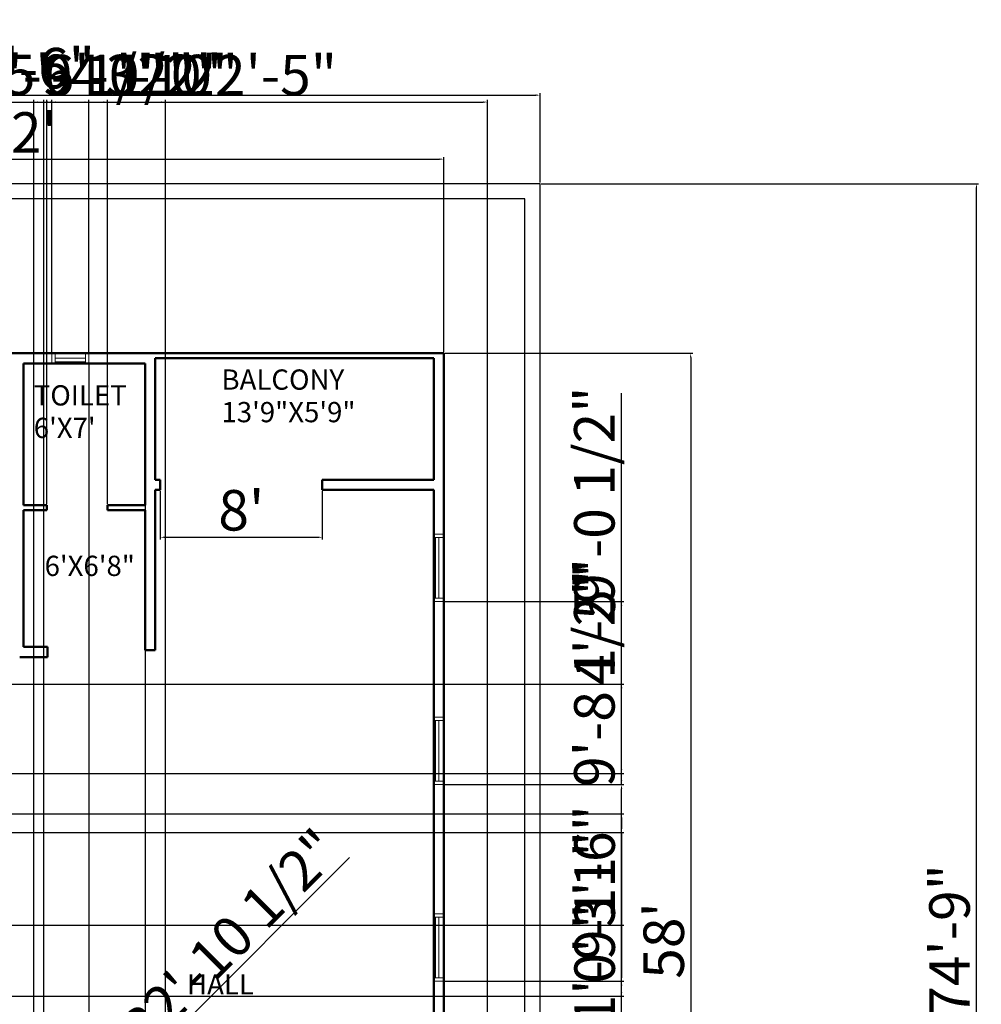
# Model space of a CAD drawing. Units: inches. Extents: x 2047 to 3023, y 479 to 1545.
# Tile 3 of 3: x 2454 to 3023, y 961 to 1545. Entities that reach past the tile are written whole.
import ezdxf

# ---------------------------------------------------------------- set-up
doc = ezdxf.new("R2010")
doc.units = ezdxf.units.IN
for name, color, linetype, lineweight in [('A-ANNO-DIMS', 2, 'Continuous', 18), ('A-AREA-IDEN', 7, 'Continuous', 25), ('A-GLAZ', 4, 'Continuous', 18), ('A-WALL', 7, 'Continuous', 50), ('C-PROP', 8, 'Continuous', 30)]:
    doc.layers.add(name, color=color, linetype=linetype, lineweight=lineweight)
doc.styles.get("Standard").update_dxf_attribs({"font": 'arial.ttf'})
doc.dimstyles.new('ISO-25', dxfattribs={"dimtxt": 24, "dimasz": 2.5, "dimexe": 1.25, "dimexo": 0.625, "dimtad": 1, "dimdec": 1, "dimlunit": 3, "dimtxsty": 'Standard', "dimcen": 2.5, "dimadec": 0, "dimazin": 0, "dimtfac": 1, "dimtdec": 1, "dimtmove": 0, "dimatfit": 3, "dimfxl": 1, "dimarcsym": 0})

# ---------------------------------------------------------------- blocks, each defined once
blk = doc.blocks.new('*D3')
at = {"layer": 'A-ANNO-DIMS', "color": 0, "lineweight": -2, "transparency": 16777216}
for p, q in [((2762.53, 1447.48), (3021.8, 1447.48)), ((3020.55, 552.98), (3020.55, 1444.98)), ((2762.53, 550.48), (3021.8, 550.48))]:
    blk.add_line(p, q, dxfattribs=at)
at = {"layer": 'A-ANNO-DIMS', "color": 0, "transparency": 16777216}
for points in [[(3020.13, 1444.98), (3020.96, 1444.98), (3020.55, 1447.48)], [(3020.13, 552.98), (3020.96, 552.98), (3020.55, 550.48)]]:
    blk.add_solid(points, dxfattribs=at)
at = {"layer": 'Defpoints', "color": 0, "transparency": 16777216}
for p in [(2761.91, 1447.48), (3020.55, 1447.48), (2761.91, 550.48)]:
    blk.add_point(p, dxfattribs=at)
at = {"layer": 'A-ANNO-DIMS', "color": 0, "transparency": 16777216, "insert": (3007.67, 998.98), "char_height": 24, "attachment_point": 5, "rotation": 90}
blk.add_mtext('74\'-9"', dxfattribs=at)
blk = doc.blocks.new('*D4')
at = {"layer": 'A-ANNO-DIMS', "color": 0, "lineweight": -2, "transparency": 16777216}
for p, q in [((2143.91, 1448.11), (2143.91, 1501.19)), ((2146.41, 1499.94), (2759.41, 1499.94)), ((2761.91, 1448.11), (2761.91, 1501.19))]:
    blk.add_line(p, q, dxfattribs=at)
at = {"layer": 'A-ANNO-DIMS', "color": 0, "transparency": 16777216}
for points in [[(2146.41, 1500.36), (2146.41, 1499.52), (2143.91, 1499.94)], [(2759.41, 1500.36), (2759.41, 1499.52), (2761.91, 1499.94)]]:
    blk.add_solid(points, dxfattribs=at)
at = {"layer": 'Defpoints', "color": 0, "transparency": 16777216}
for p in [(2761.91, 1499.94), (2143.91, 1447.48), (2761.91, 1447.48)]:
    blk.add_point(p, dxfattribs=at)
at = {"layer": 'A-ANNO-DIMS', "color": 0, "transparency": 16777216, "insert": (2452.91, 1512.82), "char_height": 24, "attachment_point": 5}
blk.add_mtext('51\'-6"', dxfattribs=at)
blk = doc.blocks.new('*D5')
at = {"layer": 'A-ANNO-DIMS', "color": 0, "lineweight": -2, "transparency": 16777216}
for p, q in [((2200.91, 1347.61), (2200.91, 1463.28)), ((2203.41, 1462.03), (2702.41, 1462.03)), ((2704.91, 1347.61), (2704.91, 1463.28))]:
    blk.add_line(p, q, dxfattribs=at)
at = {"layer": 'A-ANNO-DIMS', "color": 0, "transparency": 16777216}
for points in [[(2203.41, 1462.44), (2203.41, 1461.61), (2200.91, 1462.03)], [(2702.41, 1462.44), (2702.41, 1461.61), (2704.91, 1462.03)]]:
    blk.add_solid(points, dxfattribs=at)
at = {"layer": 'Defpoints', "color": 0, "transparency": 16777216}
for p in [(2704.91, 1462.03), (2200.91, 1346.98), (2704.91, 1346.98)]:
    blk.add_point(p, dxfattribs=at)
at = {"layer": 'A-ANNO-DIMS', "color": 0, "transparency": 16777216, "insert": (2452.91, 1474.7), "char_height": 24, "attachment_point": 5}
blk.add_mtext("42'", dxfattribs=at)
blk = doc.blocks.new('*D6')
at = {"layer": 'A-ANNO-DIMS', "color": 0, "lineweight": -2, "transparency": 16777216}
for p, q in [((2705.53, 1346.98), (2852.44, 1346.98)), ((2851.19, 1344.48), (2851.19, 653.48)), ((2705.53, 650.98), (2852.44, 650.98))]:
    blk.add_line(p, q, dxfattribs=at)
at = {"layer": 'A-ANNO-DIMS', "color": 0, "transparency": 16777216}
for points in [[(2850.77, 1344.48), (2851.6, 1344.48), (2851.19, 1346.98)], [(2850.77, 653.48), (2851.6, 653.48), (2851.19, 650.98)]]:
    blk.add_solid(points, dxfattribs=at)
at = {"layer": 'Defpoints', "color": 0, "transparency": 16777216}
for p in [(2704.91, 1346.98), (2704.91, 650.98), (2851.19, 650.98)]:
    blk.add_point(p, dxfattribs=at)
at = {"layer": 'A-ANNO-DIMS', "color": 0, "transparency": 16777216, "insert": (2838.31, 998.98), "char_height": 24, "attachment_point": 5, "rotation": 90}
blk.add_mtext("58'", dxfattribs=at)
blk = doc.blocks.new('*D9')
at = {"layer": 'A-ANNO-DIMS', "color": 0, "lineweight": -2, "transparency": 16777216}
for p, q in [((2536.91, 1265.36), (2536.91, 1236.68)), ((2632.91, 1265.36), (2632.91, 1236.68)), ((2539.41, 1237.93), (2630.41, 1237.93))]:
    blk.add_line(p, q, dxfattribs=at)
at = {"layer": 'A-ANNO-DIMS', "color": 0, "transparency": 16777216}
for points in [[(2539.41, 1238.35), (2539.41, 1237.52), (2536.91, 1237.93)], [(2630.41, 1238.35), (2630.41, 1237.52), (2632.91, 1237.93)]]:
    blk.add_solid(points, dxfattribs=at)
at = {"layer": 'Defpoints', "color": 0, "transparency": 16777216}
for p in [(2536.91, 1265.98), (2632.91, 1265.98), (2632.91, 1237.93)]:
    blk.add_point(p, dxfattribs=at)
at = {"layer": 'A-ANNO-DIMS', "color": 0, "transparency": 16777216, "insert": (2584.91, 1250.81), "char_height": 24, "attachment_point": 5}
blk.add_mtext("8'", dxfattribs=at)
blk = doc.blocks.new('WIN-36IN-6IN-FRAME')
for p, q in [((0, 6), (0, 0)), ((38, 6), (2, 6)), ((2, 6), (2, 0)), ((38, 0), (38, 6)), ((40, 0), (40, 6)), ((38, 5), (2, 5)), ((38, 3), (2, 3)), ((2, 0), (38, 0))]:
    blk.add_line(p, q)
blk = doc.blocks.new('*D24')
at = {"layer": 'A-ANNO-DIMS', "color": 0, "lineweight": -2, "transparency": 16777216}
for p, q in [((2461.91, 594.24), (2461.91, 1497.08)), ((2464.41, 1495.83), (2728.27, 1495.83)), ((2730.77, 594.24), (2730.77, 1497.08))]:
    blk.add_line(p, q, dxfattribs=at)
at = {"layer": 'A-ANNO-DIMS', "color": 0, "transparency": 16777216}
for points in [[(2464.41, 1496.25), (2464.41, 1495.41), (2461.91, 1495.83)], [(2728.27, 1496.25), (2728.27, 1495.41), (2730.77, 1495.83)]]:
    blk.add_solid(points, dxfattribs=at)
at = {"layer": 'Defpoints', "color": 0, "transparency": 16777216}
for p in [(2730.77, 1495.83), (2461.91, 593.62), (2730.77, 593.62)]:
    blk.add_point(p, dxfattribs=at)
at = {"layer": 'A-ANNO-DIMS', "color": 0, "transparency": 16777216, "insert": (2596.34, 1508.71), "char_height": 24, "attachment_point": 5}
blk.add_mtext('22\'-5"', dxfattribs=at)
blk = doc.blocks.new('*D32')
at = {"layer": 'A-ANNO-DIMS', "color": 0, "lineweight": -2, "transparency": 16777216}
for p, q in [((2705.53, 974.8), (2811.51, 974.8)), ((2810.26, 863.48), (2810.26, 972.3)), ((2699.53, 860.98), (2811.51, 860.98))]:
    blk.add_line(p, q, dxfattribs=at)
at = {"layer": 'A-ANNO-DIMS', "color": 0, "transparency": 16777216}
for points in [[(2809.84, 972.3), (2810.67, 972.3), (2810.26, 974.8)], [(2809.84, 863.48), (2810.67, 863.48), (2810.26, 860.98)]]:
    blk.add_solid(points, dxfattribs=at)
at = {"layer": 'Defpoints', "color": 0, "transparency": 16777216}
for p in [(2704.91, 974.8), (2810.26, 974.8), (2698.91, 860.98)]:
    blk.add_point(p, dxfattribs=at)
at = {"layer": 'A-ANNO-DIMS', "color": 0, "transparency": 16777216, "insert": (2797.38, 917.89), "char_height": 24, "attachment_point": 5, "rotation": 90}
blk.add_mtext('9\'-6"', dxfattribs=at)
blk = doc.blocks.new('*D33')
at = {"layer": 'A-ANNO-DIMS', "color": 0, "lineweight": -2, "transparency": 16777216}
for p, q in [((2810.26, 1091.4), (2810.26, 1214.87)), ((2705.53, 1091.4), (2811.51, 1091.4)), ((2810.26, 977.3), (2810.26, 1088.9)), ((2705.53, 974.8), (2811.51, 974.8))]:
    blk.add_line(p, q, dxfattribs=at)
at = {"layer": 'A-ANNO-DIMS', "color": 0, "transparency": 16777216}
for points in [[(2809.84, 1088.9), (2810.67, 1088.9), (2810.26, 1091.4)], [(2809.84, 977.3), (2810.67, 977.3), (2810.26, 974.8)]]:
    blk.add_solid(points, dxfattribs=at)
at = {"layer": 'Defpoints', "color": 0, "transparency": 16777216}
for p in [(2704.91, 1091.4), (2810.26, 1091.4), (2704.91, 974.8)]:
    blk.add_point(p, dxfattribs=at)
at = {"layer": 'A-ANNO-DIMS', "color": 0, "transparency": 16777216, "insert": (2797.22, 1154.38), "char_height": 24, "attachment_point": 5, "rotation": 90}
blk.add_mtext('9\'-8 1/2"', dxfattribs=at)
blk = doc.blocks.new('*D34')
at = {"layer": 'A-ANNO-DIMS', "color": 0, "lineweight": -2, "transparency": 16777216}
for p, q in [((2810.26, 1199.82), (2810.26, 1323.3)), ((2705.53, 1199.82), (2811.51, 1199.82)), ((2810.26, 1093.9), (2810.26, 1197.32)), ((2705.53, 1091.4), (2811.51, 1091.4))]:
    blk.add_line(p, q, dxfattribs=at)
at = {"layer": 'A-ANNO-DIMS', "color": 0, "transparency": 16777216}
for points in [[(2809.84, 1197.32), (2810.67, 1197.32), (2810.26, 1199.82)], [(2809.84, 1093.9), (2810.67, 1093.9), (2810.26, 1091.4)]]:
    blk.add_solid(points, dxfattribs=at)
at = {"layer": 'Defpoints', "color": 0, "transparency": 16777216}
for p in [(2704.91, 1199.82), (2810.26, 1199.82), (2704.91, 1091.4)]:
    blk.add_point(p, dxfattribs=at)
at = {"layer": 'A-ANNO-DIMS', "color": 0, "transparency": 16777216, "insert": (2797.22, 1262.81), "char_height": 24, "attachment_point": 5, "rotation": 90}
blk.add_mtext('9\'-0 1/2"', dxfattribs=at)
blk = doc.blocks.new('*D38')
at = {"layer": 'A-ANNO-DIMS', "color": 0, "lineweight": -2, "transparency": 16777216}
for p, q in [((2494.55, 1340.36), (2494.55, 500.88)), ((2527.91, 1340.36), (2527.91, 500.88)), ((2497.05, 502.13), (2525.41, 502.13)), ((2527.91, 502.13), (2651.79, 502.13))]:
    blk.add_line(p, q, dxfattribs=at)
at = {"layer": 'A-ANNO-DIMS', "color": 0, "transparency": 16777216}
for points in [[(2497.05, 502.55), (2497.05, 501.71), (2494.55, 502.13)], [(2525.41, 502.55), (2525.41, 501.71), (2527.91, 502.13)]]:
    blk.add_solid(points, dxfattribs=at)
at = {"layer": 'Defpoints', "color": 0, "transparency": 16777216}
for p in [(2494.55, 1340.98), (2527.91, 1340.98), (2527.91, 502.13)]:
    blk.add_point(p, dxfattribs=at)
at = {"layer": 'A-ANNO-DIMS', "color": 0, "transparency": 16777216, "insert": (2591.1, 515.16), "char_height": 24, "attachment_point": 5}
blk.add_mtext('2\'-9 1/2"', dxfattribs=at)
blk = doc.blocks.new('*D39')
at = {"layer": 'A-ANNO-DIMS', "color": 0, "lineweight": -2, "transparency": 16777216}
for p, q in [((2472.55, 1347.61), (2472.55, 1497.08)), ((2475.05, 1495.83), (2492.05, 1495.83)), ((2494.55, 1347.61), (2494.55, 1497.08)), ((2494.55, 1495.83), (2578.49, 1495.83))]:
    blk.add_line(p, q, dxfattribs=at)
at = {"layer": 'A-ANNO-DIMS', "color": 0, "transparency": 16777216}
for points in [[(2475.05, 1496.25), (2475.05, 1495.41), (2472.55, 1495.83)], [(2492.05, 1496.25), (2492.05, 1495.41), (2494.55, 1495.83)]]:
    blk.add_solid(points, dxfattribs=at)
at = {"layer": 'Defpoints', "color": 0, "transparency": 16777216}
for p in [(2494.55, 1495.83), (2472.55, 1346.98), (2494.55, 1346.98)]:
    blk.add_point(p, dxfattribs=at)
at = {"layer": 'A-ANNO-DIMS', "color": 0, "transparency": 16777216, "insert": (2537.77, 1508.71), "char_height": 24, "attachment_point": 5}
blk.add_mtext('1\'-10"', dxfattribs=at)
blk = doc.blocks.new('*D41')
at = {"layer": 'A-ANNO-DIMS', "color": 0, "lineweight": -2, "transparency": 16777216}
for p, q in [((2381.88, 867.61), (2381.88, 1497.08)), ((2384.38, 1495.83), (2443.66, 1495.83)), ((2446.16, 867.61), (2446.16, 1497.08)), ((2446.16, 1495.83), (2569.64, 1495.83))]:
    blk.add_line(p, q, dxfattribs=at)
at = {"layer": 'A-ANNO-DIMS', "color": 0, "transparency": 16777216}
for points in [[(2384.38, 1496.25), (2384.38, 1495.41), (2381.88, 1495.83)], [(2443.66, 1496.25), (2443.66, 1495.41), (2446.16, 1495.83)]]:
    blk.add_solid(points, dxfattribs=at)
at = {"layer": 'Defpoints', "color": 0, "transparency": 16777216}
for p in [(2446.16, 1495.83), (2381.88, 866.98), (2446.16, 866.98)]:
    blk.add_point(p, dxfattribs=at)
at = {"layer": 'A-ANNO-DIMS', "color": 0, "transparency": 16777216, "insert": (2509.15, 1508.86), "char_height": 24, "attachment_point": 5}
blk.add_mtext('5\'-4 1/2"', dxfattribs=at)
blk = doc.blocks.new('*D42')
at = {"layer": 'A-ANNO-DIMS', "color": 0, "lineweight": -2, "transparency": 16777216}
for p, q in [((2810.26, 950.97), (2810.26, 1016.25)), ((2362.53, 950.97), (2811.51, 950.97)), ((2810.26, 932.42), (2810.26, 948.47)), ((2362.53, 929.92), (2811.51, 929.92))]:
    blk.add_line(p, q, dxfattribs=at)
at = {"layer": 'A-ANNO-DIMS', "color": 0, "transparency": 16777216}
for points in [[(2809.84, 948.47), (2810.67, 948.47), (2810.26, 950.97)], [(2809.84, 932.42), (2810.67, 932.42), (2810.26, 929.92)]]:
    blk.add_solid(points, dxfattribs=at)
at = {"layer": 'Defpoints', "color": 0, "transparency": 16777216}
for p in [(2361.91, 950.97), (2810.26, 950.97), (2361.91, 929.92)]:
    blk.add_point(p, dxfattribs=at)
at = {"layer": 'A-ANNO-DIMS', "color": 0, "transparency": 16777216, "insert": (2797.38, 984.86), "char_height": 24, "attachment_point": 5, "rotation": 90}
blk.add_mtext('1\'-9"', dxfattribs=at)
blk = doc.blocks.new('*D46')
at = {"layer": 'A-ANNO-DIMS', "color": 0, "lineweight": -2, "transparency": 16777216}
for p, q in [((2810.26, 1007.98), (2810.26, 1075.51)), ((2360.53, 1007.98), (2811.51, 1007.98)), ((2810.26, 968.48), (2810.26, 1005.48)), ((2360.53, 965.98), (2811.51, 965.98))]:
    blk.add_line(p, q, dxfattribs=at)
at = {"layer": 'A-ANNO-DIMS', "color": 0, "transparency": 16777216}
for points in [[(2809.84, 1005.48), (2810.67, 1005.48), (2810.26, 1007.98)], [(2809.84, 968.48), (2810.67, 968.48), (2810.26, 965.98)]]:
    blk.add_solid(points, dxfattribs=at)
at = {"layer": 'Defpoints', "color": 0, "transparency": 16777216}
for p in [(2359.91, 1007.98), (2810.26, 1007.98), (2359.91, 965.98)]:
    blk.add_point(p, dxfattribs=at)
at = {"layer": 'A-ANNO-DIMS', "color": 0, "transparency": 16777216, "insert": (2797.37, 1043), "char_height": 24, "attachment_point": 5, "rotation": 90}
blk.add_mtext('3\'-6"', dxfattribs=at)
blk = doc.blocks.new('*D47')
at = {"layer": 'A-ANNO-DIMS', "color": 0, "lineweight": -2, "transparency": 16777216}
for p, q in [((2810.26, 1150.98), (2810.26, 1219.49)), ((2294.53, 1150.98), (2811.51, 1150.98)), ((2810.26, 1100.48), (2810.26, 1148.48)), ((2294.53, 1097.98), (2811.51, 1097.98))]:
    blk.add_line(p, q, dxfattribs=at)
at = {"layer": 'A-ANNO-DIMS', "color": 0, "transparency": 16777216}
for points in [[(2809.84, 1148.48), (2810.67, 1148.48), (2810.26, 1150.98)], [(2809.84, 1100.48), (2810.67, 1100.48), (2810.26, 1097.98)]]:
    blk.add_solid(points, dxfattribs=at)
at = {"layer": 'Defpoints', "color": 0, "transparency": 16777216}
for p in [(2293.91, 1150.98), (2810.26, 1150.98), (2293.91, 1097.98)]:
    blk.add_point(p, dxfattribs=at)
at = {"layer": 'A-ANNO-DIMS', "color": 0, "transparency": 16777216, "insert": (2797.43, 1186.49), "char_height": 24, "attachment_point": 5, "rotation": 90}
blk.add_mtext('4\'-5"', dxfattribs=at)
blk = doc.blocks.new('*D49')
at = {"layer": 'A-ANNO-DIMS', "color": 0, "lineweight": -2, "transparency": 16777216}
for p, q in [((2250.53, 1073.98), (2811.51, 1073.98)), ((2810.26, 1071.48), (2810.26, 1065.48)), ((2250.53, 1062.98), (2811.51, 1062.98)), ((2810.26, 1062.98), (2810.26, 976.79))]:
    blk.add_line(p, q, dxfattribs=at)
at = {"layer": 'A-ANNO-DIMS', "color": 0, "transparency": 16777216}
for points in [[(2809.84, 1071.48), (2810.67, 1071.48), (2810.26, 1073.98)], [(2809.84, 1065.48), (2810.67, 1065.48), (2810.26, 1062.98)]]:
    blk.add_solid(points, dxfattribs=at)
at = {"layer": 'Defpoints', "color": 0, "transparency": 16777216}
for p in [(2249.91, 1073.98), (2249.91, 1062.98), (2810.26, 1062.98)]:
    blk.add_point(p, dxfattribs=at)
at = {"layer": 'A-ANNO-DIMS', "color": 0, "transparency": 16777216, "insert": (2797.38, 1018.63), "char_height": 24, "attachment_point": 5, "rotation": 90}
blk.add_mtext('0\'-11"', dxfattribs=at)
blk = doc.blocks.new('*D50')
at = {"layer": 'A-ANNO-DIMS', "color": 0, "lineweight": -2, "transparency": 16777216}
for p, q in [((2311.99, 1173.61), (2311.99, 1497.08)), ((2314.49, 1495.83), (2427.04, 1495.83)), ((2429.54, 1173.61), (2429.54, 1497.08)), ((2429.54, 1495.83), (2553.01, 1495.83))]:
    blk.add_line(p, q, dxfattribs=at)
at = {"layer": 'A-ANNO-DIMS', "color": 0, "transparency": 16777216}
for points in [[(2314.49, 1496.25), (2314.49, 1495.41), (2311.99, 1495.83)], [(2427.04, 1496.25), (2427.04, 1495.41), (2429.54, 1495.83)]]:
    blk.add_solid(points, dxfattribs=at)
at = {"layer": 'Defpoints', "color": 0, "transparency": 16777216}
for p in [(2429.54, 1495.83), (2311.99, 1172.98), (2429.54, 1172.98)]:
    blk.add_point(p, dxfattribs=at)
at = {"layer": 'A-ANNO-DIMS', "color": 0, "transparency": 16777216, "insert": (2492.53, 1508.86), "char_height": 24, "attachment_point": 5}
blk.add_mtext('9\'-9 1/2"', dxfattribs=at)
blk = doc.blocks.new('*D51')
at = {"layer": 'A-ANNO-DIMS', "color": 0, "lineweight": -2, "transparency": 16777216}
for p, q in [((2467.91, 903.61), (2467.91, 1497.08)), ((2470.41, 1495.83), (2537.41, 1495.83)), ((2539.91, 903.61), (2539.91, 1497.08))]:
    blk.add_line(p, q, dxfattribs=at)
at = {"layer": 'A-ANNO-DIMS', "color": 0, "transparency": 16777216}
for points in [[(2470.41, 1496.25), (2470.41, 1495.41), (2467.91, 1495.83)], [(2537.41, 1496.25), (2537.41, 1495.41), (2539.91, 1495.83)]]:
    blk.add_solid(points, dxfattribs=at)
at = {"layer": 'Defpoints', "color": 0, "transparency": 16777216}
for p in [(2539.91, 1495.83), (2467.91, 902.98), (2539.91, 902.98)]:
    blk.add_point(p, dxfattribs=at)
at = {"layer": 'A-ANNO-DIMS', "color": 0, "transparency": 16777216, "insert": (2503.91, 1508.71), "char_height": 24, "attachment_point": 5}
blk.add_mtext('6\'-0"', dxfattribs=at)
blk = doc.blocks.new('*D52')
at = {"layer": 'A-ANNO-DIMS', "color": 0, "lineweight": -2, "transparency": 16777216}
for p, q in [((2469.68, 1257.61), (2469.68, 1497.08)), ((2472.18, 1495.83), (2503.18, 1495.83)), ((2505.68, 1257.61), (2505.68, 1497.08)), ((2505.68, 1495.83), (2573.21, 1495.83))]:
    blk.add_line(p, q, dxfattribs=at)
at = {"layer": 'A-ANNO-DIMS', "color": 0, "transparency": 16777216}
for points in [[(2472.18, 1496.25), (2472.18, 1495.41), (2469.68, 1495.83)], [(2503.18, 1496.25), (2503.18, 1495.41), (2505.68, 1495.83)]]:
    blk.add_solid(points, dxfattribs=at)
at = {"layer": 'Defpoints', "color": 0, "transparency": 16777216}
for p in [(2505.68, 1495.83), (2469.68, 1256.98), (2505.68, 1256.98)]:
    blk.add_point(p, dxfattribs=at)
at = {"layer": 'A-ANNO-DIMS', "color": 0, "transparency": 16777216, "insert": (2540.69, 1508.72), "char_height": 24, "attachment_point": 5}
blk.add_mtext('3\'-0"', dxfattribs=at)
blk = doc.blocks.new('*D54')
at = {"layer": 'A-ANNO-DIMS', "color": 0, "lineweight": -2, "transparency": 16777216}
for p, q in [((2649.08, 1048.15), (2495.59, 894.67)), ((2469.41, 868.48), (2493.83, 892.9))]:
    blk.add_line(p, q, dxfattribs=at)
at = {"layer": 'A-ANNO-DIMS', "color": 0, "transparency": 16777216}
blk.add_solid([(2495.3, 894.96), (2495.89, 894.37), (2493.83, 892.9)], dxfattribs=at)
at = {"layer": 'Defpoints', "color": 0, "transparency": 16777216}
for p in [(2493.83, 892.9), (2469.41, 868.48)]:
    blk.add_point(p, dxfattribs=at)
at = {"layer": 'A-ANNO-DIMS', "color": 0, "transparency": 16777216, "insert": (2564.01, 981.51), "char_height": 24, "attachment_point": 5, "rotation": 44.99969}
blk.add_mtext('2X R2\'-10 1/2"', dxfattribs=at)

msp = doc.modelspace()

# ---------------------------------------------------------------- linework, layer by layer
at = {"layer": 'A-GLAZ'}
for p, q in [((2472.55, 1346.98), (2472.55, 1340.98)), ((2492.55, 1346.98), (2474.55, 1346.98)), ((2474.55, 1346.98), (2474.55, 1340.98)), ((2492.55, 1343.98), (2474.55, 1343.98)), ((2492.55, 1340.98), (2492.55, 1346.98)), ((2494.55, 1340.98), (2494.55, 1346.98)), ((2492.55, 1341.98), (2474.55, 1341.98)), ((2474.55, 1340.98), (2492.55, 1340.98))]:
    msp.add_line(p, q, dxfattribs=at)
at = {"layer": 'A-WALL'}
for p, q in [((2704.91, 1346.98), (2248.87, 1346.98)), ((2698.91, 1343.98), (2533.91, 1343.98)), ((2533.91, 1271.98), (2533.91, 1343.98)), ((2698.91, 1271.98), (2698.91, 1343.98)), ((2704.91, 650.98), (2704.91, 1346.98)), ((2527.91, 1340.98), (2455.91, 1340.98)), ((2455.91, 1256.98), (2455.91, 1340.98)), ((2455.91, 1256.98), (2455.91, 1340.98)), ((2527.91, 1256.98), (2527.91, 1340.98)), ((2536.91, 1271.98), (2533.91, 1271.98)), ((2536.91, 1271.98), (2536.91, 1265.98)), ((2698.91, 1271.98), (2632.91, 1271.98)), ((2632.91, 1271.98), (2632.91, 1265.98)), ((2533.91, 1170.98), (2533.91, 1265.98)), ((2536.91, 1265.98), (2533.91, 1265.98)), ((2698.91, 1265.98), (2632.91, 1265.98)), ((2698.91, 866.98), (2698.91, 1265.98)), ((2469.68, 1256.98), (2455.91, 1256.98)), ((2469.68, 1256.98), (2469.68, 1253.98)), ((2527.91, 1256.98), (2505.68, 1256.98)), ((2505.68, 1256.98), (2505.68, 1253.98)), ((2455.91, 1172.98), (2455.91, 1253.98)), ((2469.68, 1253.98), (2455.91, 1253.98)), ((2527.91, 1253.98), (2505.68, 1253.98)), ((2527.91, 1173.98), (2527.91, 1253.98)), ((2470.07, 1172.98), (2455.91, 1172.98)), ((2470.07, 1172.98), (2470.07, 1170.98)), ((2527.91, 1173.98), (2527.91, 1170.98)), ((2470.07, 1170.98), (2470.07, 1166.97)), ((2527.91, 1170.98), (2533.91, 1170.98)), ((2453.57, 1166.97), (2470.07, 1166.97))]:
    msp.add_line(p, q, dxfattribs=at)
at = {"layer": 'C-PROP'}
for points in [[(2692.81, 550.48), (2761.91, 550.48), (2761.91, 1447.48), (2143.91, 1447.48), (2143.91, 550.48), (2554.81, 550.48)], [(2692.81, 559.48), (2752.91, 559.48), (2752.91, 1438.48), (2152.91, 1438.48), (2152.91, 559.48), (2554.81, 559.48)]]:
    msp.add_lwpolyline(points, dxfattribs=at)

# ---------------------------------------------------------------- block references
at = {"layer": 'A-GLAZ'}
for p, rotation in [((2704.91, 1199.82), 90.00000000000095), ((2704.91, 1091.4), 90.00000000000115), ((2704.91, 974.8), 90.00000000000115)]:
    msp.add_blockref('WIN-36IN-6IN-FRAME', p, dxfattribs=dict(at, rotation=rotation))

# ---------------------------------------------------------------- texts
at = {"layer": 'A-AREA-IDEN'}
for s, p in [('BALCONY', (2573.13, 1325.38)), ('TOILET', (2461.92, 1316.03)), ('13\'9"X5\'9"', (2573.13, 1306.1)), ("6'X7'", (2461.92, 1296.76)), ('6\'X6\'8"', (2468.34, 1214.99)), ('HALL', (2552.73, 967.01))]:
    msp.add_text(s, height=12, dxfattribs=at).set_placement(p)

# ---------------------------------------------------------------- dimensions: what is measured, and where the dimension line sits
at = {"layer": 'A-ANNO-DIMS'}
for base, p1, p2, override, picture, middle in [((2429.5398, 1495.8302), (2311.9877, 1172.9802), (2429.5398, 1172.9802), {"dimdec": 1, "dimlfac": 1, "dimrnd": 0, "dimzin": 1, "dimdsep": 46, "dimlunit": 4, "dimfrac": 2}, '*D50', (2492.5257, 1508.8645)), ((2446.16, 1495.83), (2381.88, 866.98), (2446.16, 866.98), {"dimdec": 1, "dimlfac": 1, "dimrnd": 0, "dimzin": 1, "dimdsep": 46, "dimlunit": 4, "dimfrac": 2}, '*D41', (2509.15, 1508.86)), ((2761.91, 1499.94), (2143.91, 1447.48), (2761.91, 1447.48), {"dimclrd": 0, "dimclre": 0, "dimclrt": 0}, '*D4', (2452.91, 1512.82)), ((2730.77, 1495.83), (2461.91, 593.62), (2730.77, 593.62), {"dimdec": 1, "dimlfac": 1, "dimrnd": 0, "dimzin": 1, "dimdsep": 46, "dimlunit": 4, "dimfrac": 2}, '*D24', (2596.34, 1508.71)), ((2539.91, 1495.83), (2467.91, 902.98), (2539.91, 902.98), {"dimdec": 1, "dimlfac": 1, "dimrnd": 0, "dimzin": 1, "dimdsep": 46, "dimlunit": 4, "dimfrac": 2}, '*D51', (2503.91, 1508.71)), ((2505.68, 1495.83), (2469.68, 1256.98), (2505.68, 1256.98), {"dimdec": 1, "dimlfac": 1, "dimrnd": 0, "dimzin": 1, "dimdsep": 46, "dimlunit": 4, "dimfrac": 2}, '*D52', (2540.69, 1508.72)), ((2494.55, 1495.83), (2472.55, 1346.98), (2494.55, 1346.98), {"dimdec": 1, "dimlfac": 1, "dimrnd": 0, "dimzin": 1, "dimdsep": 46, "dimlunit": 4, "dimfrac": 2}, '*D39', (2537.77, 1508.71)), ((2704.91, 1462.03), (2200.91, 1346.98), (2704.91, 1346.98), {"dimclrd": 0, "dimclre": 0, "dimclrt": 0}, '*D5', (2452.91, 1474.7)), ((2527.91, 502.13), (2494.55, 1340.98), (2527.91, 1340.98), {"dimdec": 1, "dimlfac": 1, "dimrnd": 0, "dimzin": 1, "dimdsep": 46, "dimlunit": 4, "dimfrac": 2}, '*D38', (2591.1, 515.16)), ((2632.91, 1237.93), (2536.91, 1265.98), (2632.91, 1265.98), {"dimclrd": 0, "dimclre": 0, "dimclrt": 0}, '*D9', (2584.91, 1250.81))]:
    dim = msp.add_linear_dim(base=base, p1=p1, p2=p2, dimstyle='ISO-25', override=override, dxfattribs=at)
    dim.commit()
    dim.dimension.update_dxf_attribs({"geometry": picture, "text_midpoint": middle})
for base, p1, p2, override, picture, middle in [((3020.55, 1447.48), (2761.91, 550.48), (2761.91, 1447.48), {"dimclrd": 0, "dimclre": 0, "dimclrt": 0}, '*D3', (3007.67, 998.98)), ((2851.19, 650.98), (2704.91, 1346.98), (2704.91, 650.98), {"dimclrd": 0, "dimclre": 0, "dimclrt": 0}, '*D6', (2838.31, 998.98)), ((2810.26, 1199.82), (2704.91, 1091.4), (2704.91, 1199.82), {"dimdec": 1, "dimlfac": 1, "dimrnd": 0, "dimzin": 1, "dimdsep": 46, "dimlunit": 4, "dimfrac": 2}, '*D34', (2797.22, 1262.81)), ((2810.26, 1150.98), (2293.91, 1097.98), (2293.91, 1150.98), {"dimdec": 1, "dimlfac": 1, "dimrnd": 0, "dimzin": 1, "dimdsep": 46, "dimlunit": 4, "dimfrac": 2}, '*D47', (2797.43, 1186.49)), ((2810.26, 1091.4), (2704.91, 974.8), (2704.91, 1091.4), {"dimdec": 1, "dimlfac": 1, "dimrnd": 0, "dimzin": 1, "dimdsep": 46, "dimlunit": 4, "dimfrac": 2}, '*D33', (2797.22, 1154.38)), ((2810.26, 1062.98), (2249.91, 1073.98), (2249.91, 1062.98), {"dimdec": 1, "dimlfac": 1, "dimrnd": 0, "dimzin": 1, "dimdsep": 46, "dimlunit": 4, "dimfrac": 2}, '*D49', (2797.38, 1018.63)), ((2810.26, 1007.98), (2359.91, 965.98), (2359.91, 1007.98), {"dimdec": 1, "dimlfac": 1, "dimrnd": 0, "dimzin": 1, "dimdsep": 46, "dimlunit": 4, "dimfrac": 2}, '*D46', (2797.37, 1043)), ((2810.258, 950.966), (2361.908, 929.9219), (2361.908, 950.966), {"dimdec": 1, "dimlfac": 1, "dimrnd": 0, "dimzin": 1, "dimdsep": 46, "dimlunit": 4, "dimfrac": 2}, '*D42', (2797.3792, 984.8604)), ((2810.26, 974.8), (2698.91, 860.98), (2704.91, 974.8), {"dimdec": 1, "dimlfac": 1, "dimrnd": 0, "dimzin": 1, "dimdsep": 46, "dimlunit": 4, "dimfrac": 2}, '*D32', (2797.38, 917.89))]:
    dim = msp.add_linear_dim(base=base, p1=p1, p2=p2, angle=90, dimstyle='ISO-25', override=override, dxfattribs=at)
    dim.commit()
    dim.dimension.update_dxf_attribs({"geometry": picture, "text_midpoint": middle})
dim = msp.add_radius_dim(center=(2469.41, 868.48), mpoint=(2493.83, 892.9), text='2X <>', dimstyle='ISO-25', override={"dimdec": 1, "dimlfac": 1, "dimrnd": 0, "dimzin": 1, "dimdsep": 46, "dimlunit": 4, "dimfrac": 2}, dxfattribs=at)
dim.commit()
dim.dimension.update_dxf_attribs({"geometry": '*D54', "text_midpoint": (2564.01, 981.51)})

doc.saveas('drawing.dxf')
